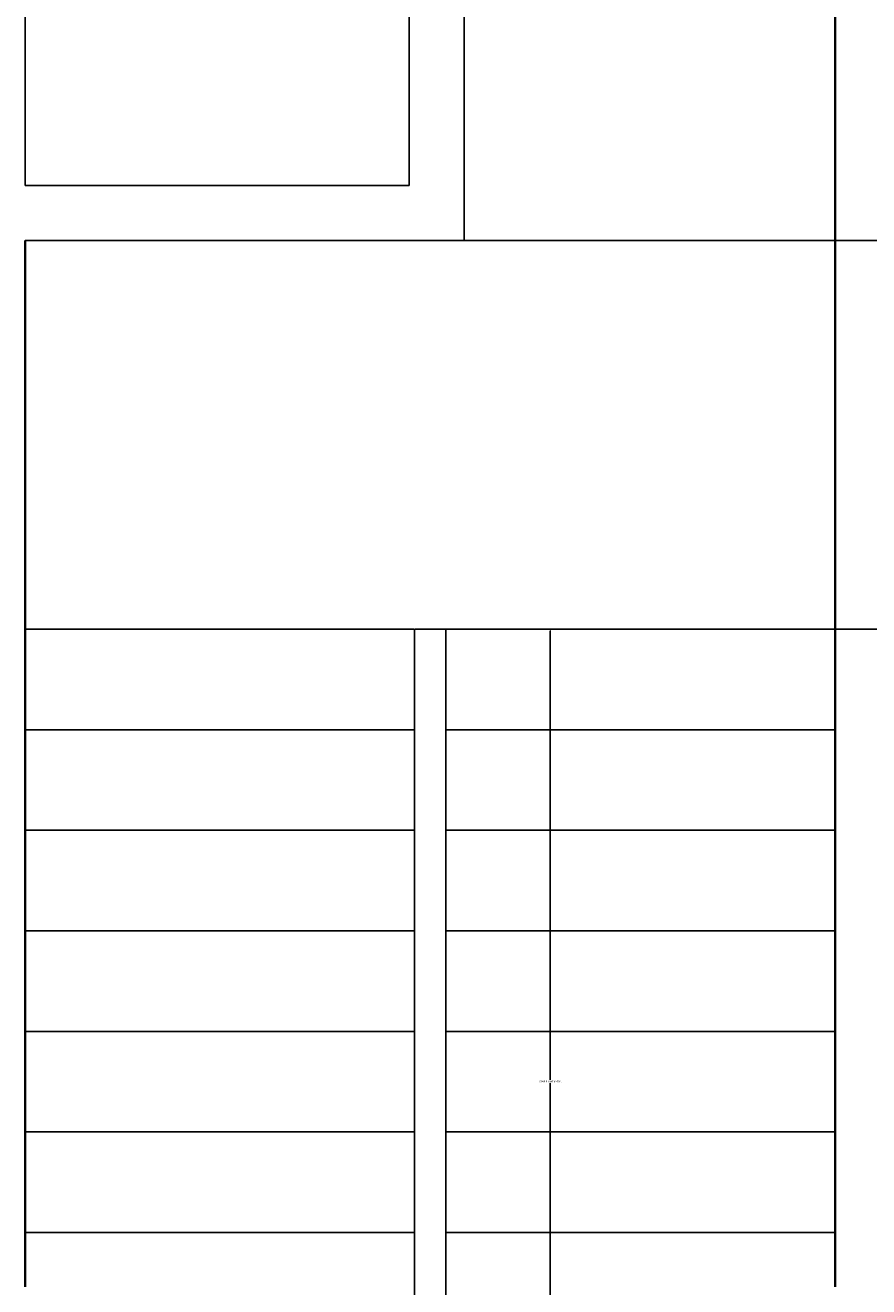
# Model space of a CAD drawing. Units: inches. Extents: x 4159 to 4826, y 299 to 1026.
# Tile 29 of 37: x 4453 to 4546, y 401 to 539. Entities that reach past the tile are written whole.
import ezdxf

# ---------------------------------------------------------------- set-up
doc = ezdxf.new("R2010")
doc.units = ezdxf.units.IN
for name, color, linetype, lineweight in [('A-ANNO-DIMS', 2, 'Continuous', 18), ('A-FLOR-EVTR', 6, 'Continuous', 25), ('A-FLOR-STRS', 3, 'Continuous', 25), ('A-WALL', 7, 'Continuous', 35)]:
    doc.layers.add(name, color=color, linetype=linetype, lineweight=lineweight)
doc.styles.get("Standard").update_dxf_attribs({"font": 'arial.ttf'})
doc.dimstyles.get("Standard").update_dxf_attribs({"dimtxt": 0.18, "dimasz": 0.18, "dimexe": 0.18, "dimexo": 0.0625, "dimgap": 0.09, "dimtad": 0, "dimtih": 1, "dimtoh": 1, "dimdec": 4, "dimzin": 0, "dimdsep": 46, "dimtxsty": 'Standard', "dimcen": 0.09, "dimadec": 0, "dimazin": 0, "dimtfac": 1, "dimtdec": 4, "dimtofl": 0, "dimtmove": 0, "dimatfit": 3, "dimfxl": 1, "dimtolj": 1, "dimtzin": 0, "dimarcsym": 0})

# ---------------------------------------------------------------- blocks, each defined once
blk = doc.blocks.new('STAIR-FLIGHT-9-TREAD')
for p, q in [((0, 99), (42.58, 99)), ((42.58, 99), (42.58, 0)), ((0, 88), (42.58, 88)), ((0, 77), (42.58, 77)), ((0, 66), (42.58, 66)), ((0, 55), (42.58, 55)), ((0, 44), (42.58, 44)), ((0, 33), (42.58, 33)), ((0, 22), (42.58, 22)), ((0, 11), (42.58, 11))]:
    blk.add_line(p, q)
blk = doc.blocks.new('*D41')
at = {"layer": 'A-ANNO-DIMS', "color": 0, "lineweight": -2, "transparency": 16777216}
for p, q in [((4495.95, 473.2), (4510.92, 473.2)), ((4510.74, 473.02), (4510.74, 423.88)), ((4510.74, 374.38), (4510.74, 423.51)), ((4495.95, 374.2), (4510.92, 374.2))]:
    blk.add_line(p, q, dxfattribs=at)
at = {"layer": 'A-ANNO-DIMS', "color": 0, "transparency": 16777216}
for points in [[(4510.71, 473.02), (4510.77, 473.02), (4510.74, 473.2)], [(4510.71, 374.38), (4510.77, 374.38), (4510.74, 374.2)]]:
    blk.add_solid(points, dxfattribs=at)
at = {"layer": 'Defpoints', "color": 0, "transparency": 16777216}
for p in [(4495.89, 473.2), (4510.74, 473.2), (4495.89, 374.2)]:
    blk.add_point(p, dxfattribs=at)
at = {"layer": 'A-ANNO-DIMS', "color": 0, "transparency": 16777216, "insert": (4510.74, 423.7), "char_height": 0.18, "attachment_point": 5}
blk.add_mtext('\\A1;STAIR FLIGHT 99 TYP.', dxfattribs=at)
blk = doc.blocks.new('*D54')
at = {"layer": 'A-ANNO-DIMS', "color": 0, "lineweight": -2, "transparency": 16777216}
for p, q in [((4501.37, 515.71), (4825.74, 515.71)), ((4825.56, 515.53), (4825.56, 494.64)), ((4825.56, 473.38), (4825.56, 494.27)), ((4541.95, 473.2), (4825.74, 473.2))]:
    blk.add_line(p, q, dxfattribs=at)
at = {"layer": 'A-ANNO-DIMS', "color": 0, "transparency": 16777216}
for points in [[(4825.53, 515.53), (4825.59, 515.53), (4825.56, 515.71)], [(4825.53, 473.38), (4825.59, 473.38), (4825.56, 473.2)]]:
    blk.add_solid(points, dxfattribs=at)
at = {"layer": 'Defpoints', "color": 0, "transparency": 16777216}
for p in [(4501.31, 515.71), (4825.56, 515.71), (4541.89, 473.2)]:
    blk.add_point(p, dxfattribs=at)
at = {"layer": 'A-ANNO-DIMS', "color": 0, "transparency": 16777216, "insert": (4825.56, 494.45), "char_height": 0.18, "attachment_point": 5}
blk.add_mtext('\\A1;42.52', dxfattribs=at)

msp = doc.modelspace()

# ---------------------------------------------------------------- linework, layer by layer
at = {"layer": 'A-FLOR-EVTR'}
for p, q in [((4501.31, 581.713), (4501.31, 515.713)), ((4453.31, 575.713), (4453.31, 521.713)), ((4495.31, 575.713), (4495.31, 521.713)), ((4453.31, 521.713), (4495.31, 521.713)), ((4453.31, 515.713), (4501.31, 515.713))]:
    msp.add_line(p, q, dxfattribs=at)
at = {"layer": 'A-WALL'}
for p, q in [((4541.889, 618.254), (4541.889, 401.254)), ((4453.31, 515.713), (4453.31, 401.254))]:
    msp.add_line(p, q, dxfattribs=at)

# ---------------------------------------------------------------- block references
at = {"layer": 'A-FLOR-STRS'}
msp.add_blockref('STAIR-FLIGHT-9-TREAD', (4453.31, 374.195), dxfattribs=at)
at = {"layer": 'A-FLOR-STRS', "extrusion": (0, 0, -1), "zscale": -1}
msp.add_blockref('STAIR-FLIGHT-9-TREAD', (-4541.889, 374.195), dxfattribs=at)

# ---------------------------------------------------------------- dimensions: what is measured, and where the dimension line sits
at = {"layer": 'A-ANNO-DIMS'}
dim = msp.add_linear_dim(base=(4825.56, 515.713), p1=(4541.889, 473.195), p2=(4501.31, 515.713), angle=90, dimstyle='Standard', override={"dimdec": 2, "dimlfac": 1, "dimrnd": 0, "dimzin": 0, "dimdsep": 46, "dimlunit": 2}, dxfattribs=at)
dim.commit()
dim.dimension.update_dxf_attribs({"geometry": '*D54', "text_midpoint": (4825.56, 494.454)})
dim = msp.add_linear_dim(base=(4510.739, 473.195), p1=(4495.889, 374.195), p2=(4495.889, 473.195), angle=90, text='STAIR FLIGHT <> TYP.', dimstyle='Standard', override={"dimdec": 0, "dimlfac": 1, "dimrnd": 0, "dimzin": 0, "dimdsep": 46, "dimlunit": 2}, dxfattribs=at)
dim.commit()
dim.dimension.update_dxf_attribs({"geometry": '*D41', "text_midpoint": (4510.739, 423.695)})

doc.saveas('drawing.dxf')
